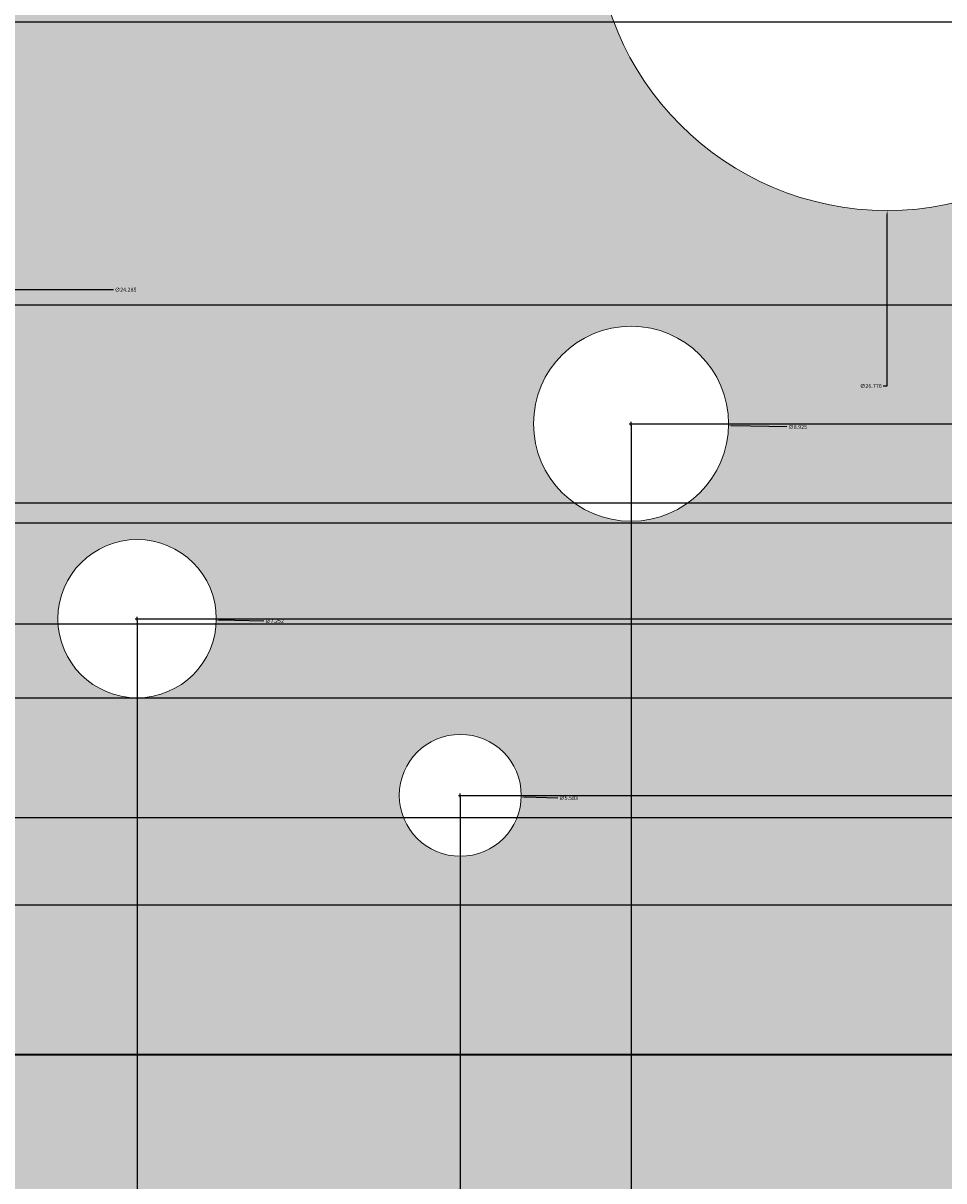
# Model space of a CAD drawing. Units: inches. Extents: x 73 to 607, y 92 to 651.
# Tile 9 of 18: x 504 to 546, y 169 to 222. Entities that reach past the tile are written whole.
import ezdxf

# ---------------------------------------------------------------- set-up
doc = ezdxf.new("R2010")
doc.units = ezdxf.units.IN
doc.header["$MEASUREMENT"] = 0
for name, color, linetype, lineweight in [('A-ANNO-DIMS', 2, 'Continuous', 18), ('A-ELEV', 7, 'Continuous', 35), ('A-ELEV-PANL', 7, 'Continuous', 18), ('A-ELEV-PATT-BKGD', 252, 'Continuous', 13), ('A-ELEV-PATT-SHAD', 8, 'Continuous', 13), ('A-ELEV-PATT-WOOD', 32, 'Continuous', 13)]:
    doc.layers.add(name, color=color, linetype=linetype, lineweight=lineweight)
doc.styles.get("Standard").update_dxf_attribs({"font": 'arial.ttf'})
doc.dimstyles.get("Standard").update_dxf_attribs({"dimtxt": 0.18, "dimasz": 0.18, "dimexe": 0.18, "dimexo": 0.0625, "dimgap": 0.09, "dimtad": 0, "dimtih": 1, "dimtoh": 1, "dimdec": 4, "dimzin": 0, "dimdsep": 46, "dimtxsty": 'Standard', "dimcen": 0.09, "dimadec": 0, "dimazin": 0, "dimtfac": 1, "dimtdec": 4, "dimtofl": 0, "dimtmove": 0, "dimatfit": 3, "dimfxl": 1, "dimtolj": 1, "dimtzin": 0, "dimarcsym": 0})

# ---------------------------------------------------------------- blocks, each defined once
blk = doc.blocks.new('*D15')
at = {"layer": 'A-ANNO-DIMS', "color": 0, "lineweight": -2, "transparency": 16777216}
for p, q in [((454.767, 174.802), (607.278, 174.802)), ((607.098, 174.622), (607.098, 159.185)), ((607.098, 143.384), (607.098, 158.821)), ((580.161, 143.204), (607.278, 143.204))]:
    blk.add_line(p, q, dxfattribs=at)
at = {"layer": 'A-ANNO-DIMS', "color": 0, "transparency": 16777216}
for points in [[(607.068, 174.622), (607.128, 174.622), (607.098, 174.802)], [(607.068, 143.384), (607.128, 143.384), (607.098, 143.204)]]:
    blk.add_solid(points, dxfattribs=at)
at = {"layer": 'Defpoints', "color": 0, "transparency": 16777216}
for p in [(454.705, 174.802), (607.098, 174.802), (580.098, 143.204)]:
    blk.add_point(p, dxfattribs=at)
at = {"layer": 'A-ANNO-DIMS', "color": 0, "transparency": 16777216, "insert": (607.098, 159.003), "char_height": 0.18, "attachment_point": 5}
blk.add_mtext('\\A1;31.6', dxfattribs=at)
blk = doc.blocks.new('*D16')
at = {"layer": 'A-ANNO-DIMS', "color": 0, "lineweight": -2, "transparency": 16777216}
for p, q in [((431.133, 185.662), (607.278, 185.662)), ((607.098, 185.482), (607.098, 180.414)), ((607.098, 174.982), (607.098, 180.05)), ((454.767, 174.802), (607.278, 174.802))]:
    blk.add_line(p, q, dxfattribs=at)
at = {"layer": 'A-ANNO-DIMS', "color": 0, "transparency": 16777216}
for points in [[(607.068, 185.482), (607.128, 185.482), (607.098, 185.662)], [(607.068, 174.982), (607.128, 174.982), (607.098, 174.802)]]:
    blk.add_solid(points, dxfattribs=at)
at = {"layer": 'Defpoints', "color": 0, "transparency": 16777216}
for p in [(431.07, 185.662), (607.098, 185.662), (454.705, 174.802)]:
    blk.add_point(p, dxfattribs=at)
at = {"layer": 'A-ANNO-DIMS', "color": 0, "transparency": 16777216, "insert": (607.098, 180.232), "char_height": 0.18, "attachment_point": 5}
blk.add_mtext('\\A1;10.86', dxfattribs=at)
blk = doc.blocks.new('*D17')
at = {"layer": 'A-ANNO-DIMS', "color": 0, "lineweight": -2, "transparency": 16777216}
for p, q in [((580.161, 262.302), (607.278, 262.302)), ((607.098, 262.122), (607.098, 224.164)), ((607.098, 185.842), (607.098, 223.8)), ((431.133, 185.662), (607.278, 185.662))]:
    blk.add_line(p, q, dxfattribs=at)
at = {"layer": 'A-ANNO-DIMS', "color": 0, "transparency": 16777216}
for points in [[(607.068, 262.122), (607.128, 262.122), (607.098, 262.302)], [(607.068, 185.842), (607.128, 185.842), (607.098, 185.662)]]:
    blk.add_solid(points, dxfattribs=at)
at = {"layer": 'Defpoints', "color": 0, "transparency": 16777216}
for p in [(580.098, 262.302), (607.098, 262.302), (431.07, 185.662)]:
    blk.add_point(p, dxfattribs=at)
at = {"layer": 'A-ANNO-DIMS', "color": 0, "transparency": 16777216, "insert": (607.098, 223.982), "char_height": 0.18, "attachment_point": 5}
blk.add_mtext('\\A1;76.64', dxfattribs=at)
blk = doc.blocks.new('*D62')
at = {"layer": 'A-ANNO-DIMS', "color": 0, "lineweight": -2, "transparency": 16777216}
for p, q in [((488.442, 209.739), (488.442, 209.919)), ((488.352, 209.829), (488.532, 209.829)), ((507.87, 209.829), (500.764, 209.829))]:
    blk.add_line(p, q, dxfattribs=at)
at = {"layer": 'A-ANNO-DIMS', "color": 0, "transparency": 16777216}
blk.add_solid([(500.764, 209.859), (500.764, 209.799), (500.584, 209.829)], dxfattribs=at)
at = {"layer": 'Defpoints', "color": 0, "transparency": 16777216}
for p in [(476.3, 209.828), (500.584, 209.829)]:
    blk.add_point(p, dxfattribs=at)
at = {"layer": 'A-ANNO-DIMS', "color": 0, "transparency": 16777216, "insert": (508.432, 209.829), "char_height": 0.18, "attachment_point": 5}
blk.add_mtext('\\A1;∅24.285', dxfattribs=at)
blk = doc.blocks.new('*D94')
at = {"layer": 'A-ANNO-DIMS', "color": 0, "lineweight": -2, "transparency": 16777216}
for p, q in [((377.023, 209.143), (607.278, 209.143)), ((607.098, 208.963), (607.098, 204.329)), ((607.098, 199.331), (607.098, 203.965)), ((363.319, 199.151), (607.278, 199.151))]:
    blk.add_line(p, q, dxfattribs=at)
at = {"layer": 'A-ANNO-DIMS', "color": 0, "transparency": 16777216}
for points in [[(607.068, 208.963), (607.128, 208.963), (607.098, 209.143)], [(607.068, 199.331), (607.128, 199.331), (607.098, 199.151)]]:
    blk.add_solid(points, dxfattribs=at)
at = {"layer": 'Defpoints', "color": 0, "transparency": 16777216}
for p in [(376.96, 209.143), (363.256, 199.151), (607.098, 199.151)]:
    blk.add_point(p, dxfattribs=at)
at = {"layer": 'A-ANNO-DIMS', "color": 0, "transparency": 16777216, "insert": (607.098, 204.147), "char_height": 0.18, "attachment_point": 5}
blk.add_mtext('\\A1;9.992', dxfattribs=at)
blk = doc.blocks.new('*D95')
at = {"layer": 'A-ANNO-DIMS', "color": 0, "lineweight": -2, "transparency": 16777216}
for p, q in [((363.874, 225.982), (607.278, 225.982)), ((607.098, 225.802), (607.098, 212.749)), ((607.098, 199.331), (607.098, 212.385)), ((363.319, 199.151), (607.278, 199.151))]:
    blk.add_line(p, q, dxfattribs=at)
at = {"layer": 'A-ANNO-DIMS', "color": 0, "transparency": 16777216}
for points in [[(607.068, 225.802), (607.128, 225.802), (607.098, 225.982)], [(607.068, 199.331), (607.128, 199.331), (607.098, 199.151)]]:
    blk.add_solid(points, dxfattribs=at)
at = {"layer": 'Defpoints', "color": 0, "transparency": 16777216}
for p in [(363.812, 225.982), (607.098, 225.982), (363.256, 199.151)]:
    blk.add_point(p, dxfattribs=at)
at = {"layer": 'A-ANNO-DIMS', "color": 0, "transparency": 16777216, "insert": (607.098, 212.567), "char_height": 0.18, "attachment_point": 5}
blk.add_mtext('\\A1;26.83', dxfattribs=at)
blk = doc.blocks.new('*D97')
at = {"layer": 'A-ANNO-DIMS', "color": 0, "lineweight": -2, "transparency": 16777216}
for p, q in [((387.579, 200.076), (607.278, 200.076)), ((607.098, 199.896), (607.098, 197.488)), ((607.098, 194.717), (607.098, 197.125)), ((396.755, 194.537), (607.278, 194.537))]:
    blk.add_line(p, q, dxfattribs=at)
at = {"layer": 'A-ANNO-DIMS', "color": 0, "transparency": 16777216}
for points in [[(607.068, 199.896), (607.128, 199.896), (607.098, 200.076)], [(607.068, 194.717), (607.128, 194.717), (607.098, 194.537)]]:
    blk.add_solid(points, dxfattribs=at)
at = {"layer": 'Defpoints', "color": 0, "transparency": 16777216}
for p in [(387.516, 200.076), (607.098, 200.076), (396.692, 194.537)]:
    blk.add_point(p, dxfattribs=at)
at = {"layer": 'A-ANNO-DIMS', "color": 0, "transparency": 16777216, "insert": (607.098, 197.306), "char_height": 0.18, "attachment_point": 5}
blk.add_mtext('\\A1;5.54', dxfattribs=at)
blk = doc.blocks.new('*D98')
at = {"layer": 'A-ANNO-DIMS', "color": 0, "lineweight": -2, "transparency": 16777216}
for p, q in [((377.023, 209.143), (607.278, 209.143)), ((607.098, 208.963), (607.098, 204.792)), ((607.098, 200.256), (607.098, 204.428)), ((387.579, 200.076), (607.278, 200.076))]:
    blk.add_line(p, q, dxfattribs=at)
at = {"layer": 'A-ANNO-DIMS', "color": 0, "transparency": 16777216}
for points in [[(607.068, 208.963), (607.128, 208.963), (607.098, 209.143)], [(607.068, 200.256), (607.128, 200.256), (607.098, 200.076)]]:
    blk.add_solid(points, dxfattribs=at)
at = {"layer": 'Defpoints', "color": 0, "transparency": 16777216}
for p in [(376.96, 209.143), (607.098, 209.143), (387.516, 200.076)]:
    blk.add_point(p, dxfattribs=at)
at = {"layer": 'A-ANNO-DIMS', "color": 0, "transparency": 16777216, "insert": (607.098, 204.61), "char_height": 0.18, "attachment_point": 5}
blk.add_mtext('\\A1;9.067', dxfattribs=at)
blk = doc.blocks.new('*D99')
at = {"layer": 'A-ANNO-DIMS', "color": 0, "lineweight": -2, "transparency": 16777216}
for p, q in [((373.319, 231.348), (607.278, 231.348)), ((607.098, 231.168), (607.098, 220.428)), ((607.098, 209.323), (607.098, 220.064)), ((377.023, 209.143), (607.278, 209.143))]:
    blk.add_line(p, q, dxfattribs=at)
at = {"layer": 'A-ANNO-DIMS', "color": 0, "transparency": 16777216}
for points in [[(607.068, 231.168), (607.128, 231.168), (607.098, 231.348)], [(607.068, 209.323), (607.128, 209.323), (607.098, 209.143)]]:
    blk.add_solid(points, dxfattribs=at)
at = {"layer": 'Defpoints', "color": 0, "transparency": 16777216}
for p in [(373.257, 231.348), (607.098, 231.348), (376.96, 209.143)]:
    blk.add_point(p, dxfattribs=at)
at = {"layer": 'A-ANNO-DIMS', "color": 0, "transparency": 16777216, "insert": (607.098, 220.246), "char_height": 0.18, "attachment_point": 5}
blk.add_mtext('\\A1;22.205', dxfattribs=at)
blk = doc.blocks.new('*D100')
at = {"layer": 'A-ANNO-DIMS', "color": 0, "lineweight": -2, "transparency": 16777216}
for p, q in [((382.949, 222.096), (607.278, 222.096)), ((607.098, 221.916), (607.098, 211.268)), ((607.098, 200.256), (607.098, 210.904)), ((387.579, 200.076), (607.278, 200.076))]:
    blk.add_line(p, q, dxfattribs=at)
at = {"layer": 'A-ANNO-DIMS', "color": 0, "transparency": 16777216}
for points in [[(607.068, 221.916), (607.128, 221.916), (607.098, 222.096)], [(607.068, 200.256), (607.128, 200.256), (607.098, 200.076)]]:
    blk.add_solid(points, dxfattribs=at)
at = {"layer": 'Defpoints', "color": 0, "transparency": 16777216}
for p in [(382.886, 222.096), (607.098, 222.096), (387.516, 200.076)]:
    blk.add_point(p, dxfattribs=at)
at = {"layer": 'A-ANNO-DIMS', "color": 0, "transparency": 16777216, "insert": (607.098, 211.086), "char_height": 0.18, "attachment_point": 5}
blk.add_mtext('\\A1;22.02', dxfattribs=at)
blk = doc.blocks.new('*D113')
at = {"layer": 'A-ANNO-DIMS', "color": 0, "lineweight": -2, "transparency": 16777216}
for p, q in [((508.958, 194.705), (508.958, 116.024)), ((492.769, 181.596), (492.769, 116.024)), ((492.949, 116.204), (500.478, 116.204)), ((508.778, 116.204), (501.249, 116.204))]:
    blk.add_line(p, q, dxfattribs=at)
at = {"layer": 'A-ANNO-DIMS', "color": 0, "transparency": 16777216}
for points in [[(492.949, 116.234), (492.949, 116.174), (492.769, 116.204)], [(508.778, 116.234), (508.778, 116.174), (508.958, 116.204)]]:
    blk.add_solid(points, dxfattribs=at)
at = {"layer": 'Defpoints', "color": 0, "transparency": 16777216}
for p in [(508.958, 194.767), (492.769, 181.659), (508.958, 116.204)]:
    blk.add_point(p, dxfattribs=at)
at = {"layer": 'A-ANNO-DIMS', "color": 0, "transparency": 16777216, "insert": (500.864, 116.204), "char_height": 0.18, "attachment_point": 5}
blk.add_mtext('\\A1;16.19', dxfattribs=at)
blk = doc.blocks.new('*D114')
at = {"layer": 'A-ANNO-DIMS', "color": 0, "lineweight": -2, "transparency": 16777216}
for p, q in [((508.958, 194.705), (508.958, 116.024)), ((523.753, 186.617), (523.753, 116.024)), ((509.138, 116.204), (515.901, 116.204)), ((523.573, 116.204), (516.81, 116.204))]:
    blk.add_line(p, q, dxfattribs=at)
at = {"layer": 'A-ANNO-DIMS', "color": 0, "transparency": 16777216}
for points in [[(509.138, 116.234), (509.138, 116.174), (508.958, 116.204)], [(523.573, 116.234), (523.573, 116.174), (523.753, 116.204)]]:
    blk.add_solid(points, dxfattribs=at)
at = {"layer": 'Defpoints', "color": 0, "transparency": 16777216}
for p in [(508.958, 194.767), (523.753, 186.679), (523.753, 116.204)]:
    blk.add_point(p, dxfattribs=at)
at = {"layer": 'A-ANNO-DIMS', "color": 0, "transparency": 16777216, "insert": (516.356, 116.204), "char_height": 0.18, "attachment_point": 5}
blk.add_mtext('\\A1;14.794', dxfattribs=at)
blk = doc.blocks.new('*D115')
at = {"layer": 'A-ANNO-DIMS', "color": 0, "lineweight": -2, "transparency": 16777216}
for p, q in [((531.568, 203.63), (531.568, 116.024)), ((523.753, 186.617), (523.753, 116.024)), ((523.933, 116.204), (527.268, 116.204)), ((531.388, 116.204), (528.053, 116.204))]:
    blk.add_line(p, q, dxfattribs=at)
at = {"layer": 'A-ANNO-DIMS', "color": 0, "transparency": 16777216}
for points in [[(523.933, 116.234), (523.933, 116.174), (523.753, 116.204)], [(531.388, 116.234), (531.388, 116.174), (531.568, 116.204)]]:
    blk.add_solid(points, dxfattribs=at)
at = {"layer": 'Defpoints', "color": 0, "transparency": 16777216}
for p in [(531.568, 203.693), (523.753, 186.679), (531.568, 116.204)]:
    blk.add_point(p, dxfattribs=at)
at = {"layer": 'A-ANNO-DIMS', "color": 0, "transparency": 16777216, "insert": (527.661, 116.204), "char_height": 0.18, "attachment_point": 5}
blk.add_mtext('\\A1;7.816', dxfattribs=at)
blk = doc.blocks.new('*D116')
at = {"layer": 'A-ANNO-DIMS', "color": 0, "lineweight": -2, "transparency": 16777216}
for p, q in [((531.568, 203.63), (531.568, 116.024)), ((550.829, 183.548), (550.829, 116.024)), ((531.748, 116.204), (540.814, 116.204)), ((550.649, 116.204), (541.584, 116.204))]:
    blk.add_line(p, q, dxfattribs=at)
at = {"layer": 'A-ANNO-DIMS', "color": 0, "transparency": 16777216}
for points in [[(531.748, 116.234), (531.748, 116.174), (531.568, 116.204)], [(550.649, 116.234), (550.649, 116.174), (550.829, 116.204)]]:
    blk.add_solid(points, dxfattribs=at)
at = {"layer": 'Defpoints', "color": 0, "transparency": 16777216}
for p in [(531.568, 203.693), (550.829, 183.611), (550.829, 116.204)]:
    blk.add_point(p, dxfattribs=at)
at = {"layer": 'A-ANNO-DIMS', "color": 0, "transparency": 16777216, "insert": (541.199, 116.204), "char_height": 0.18, "attachment_point": 5}
blk.add_mtext('\\A1;19.26', dxfattribs=at)
blk = doc.blocks.new('*D120')
at = {"layer": 'A-ANNO-DIMS', "color": 0, "lineweight": -2, "transparency": 16777216}
for p, q in [((468.546, 225.727), (607.278, 225.727)), ((607.098, 225.547), (607.098, 208.616)), ((607.098, 191.322), (607.098, 208.252)), ((469.942, 191.142), (607.278, 191.142))]:
    blk.add_line(p, q, dxfattribs=at)
at = {"layer": 'A-ANNO-DIMS', "color": 0, "transparency": 16777216}
for points in [[(607.068, 225.547), (607.128, 225.547), (607.098, 225.727)], [(607.068, 191.322), (607.128, 191.322), (607.098, 191.142)]]:
    blk.add_solid(points, dxfattribs=at)
at = {"layer": 'Defpoints', "color": 0, "transparency": 16777216}
for p in [(468.484, 225.727), (607.098, 225.727), (469.879, 191.142)]:
    blk.add_point(p, dxfattribs=at)
at = {"layer": 'A-ANNO-DIMS', "color": 0, "transparency": 16777216, "insert": (607.098, 208.434), "char_height": 0.18, "attachment_point": 5}
blk.add_mtext('\\A1;34.585', dxfattribs=at)
blk = doc.blocks.new('*D122')
at = {"layer": 'A-ANNO-DIMS', "color": 0, "lineweight": -2, "transparency": 16777216}
for p, q in [((509.021, 194.767), (607.278, 194.767)), ((607.098, 194.587), (607.098, 188.395)), ((607.098, 181.839), (607.098, 188.031)), ((492.831, 181.659), (607.278, 181.659))]:
    blk.add_line(p, q, dxfattribs=at)
at = {"layer": 'A-ANNO-DIMS', "color": 0, "transparency": 16777216}
for points in [[(607.068, 194.587), (607.128, 194.587), (607.098, 194.767)], [(607.068, 181.839), (607.128, 181.839), (607.098, 181.659)]]:
    blk.add_solid(points, dxfattribs=at)
at = {"layer": 'Defpoints', "color": 0, "transparency": 16777216}
for p in [(508.958, 194.767), (492.769, 181.659), (607.098, 181.659)]:
    blk.add_point(p, dxfattribs=at)
at = {"layer": 'A-ANNO-DIMS', "color": 0, "transparency": 16777216, "insert": (607.098, 188.213), "char_height": 0.18, "attachment_point": 5}
blk.add_mtext('\\A1;13.11', dxfattribs=at)
blk = doc.blocks.new('*D124')
at = {"layer": 'A-ANNO-DIMS', "color": 0, "lineweight": -2, "transparency": 16777216}
for p, q in [((523.815, 186.679), (607.278, 186.679)), ((607.098, 186.499), (607.098, 185.327)), ((607.098, 183.791), (607.098, 184.963)), ((550.891, 183.611), (607.278, 183.611))]:
    blk.add_line(p, q, dxfattribs=at)
at = {"layer": 'A-ANNO-DIMS', "color": 0, "transparency": 16777216}
for points in [[(607.068, 186.499), (607.128, 186.499), (607.098, 186.679)], [(607.068, 183.791), (607.128, 183.791), (607.098, 183.611)]]:
    blk.add_solid(points, dxfattribs=at)
at = {"layer": 'Defpoints', "color": 0, "transparency": 16777216}
for p in [(523.753, 186.679), (607.098, 186.679), (550.829, 183.611)]:
    blk.add_point(p, dxfattribs=at)
at = {"layer": 'A-ANNO-DIMS', "color": 0, "transparency": 16777216, "insert": (607.098, 185.145), "char_height": 0.18, "attachment_point": 5}
blk.add_mtext('\\A1;3.068', dxfattribs=at)
blk = doc.blocks.new('*D125')
at = {"layer": 'A-ANNO-DIMS', "color": 0, "lineweight": -2, "transparency": 16777216}
for p, q in [((509.021, 194.767), (607.278, 194.767)), ((607.098, 194.587), (607.098, 190.905)), ((607.098, 186.859), (607.098, 190.541)), ((523.815, 186.679), (607.278, 186.679))]:
    blk.add_line(p, q, dxfattribs=at)
at = {"layer": 'A-ANNO-DIMS', "color": 0, "transparency": 16777216}
for points in [[(607.068, 194.587), (607.128, 194.587), (607.098, 194.767)], [(607.068, 186.859), (607.128, 186.859), (607.098, 186.679)]]:
    blk.add_solid(points, dxfattribs=at)
at = {"layer": 'Defpoints', "color": 0, "transparency": 16777216}
for p in [(508.958, 194.767), (607.098, 194.767), (523.753, 186.679)]:
    blk.add_point(p, dxfattribs=at)
at = {"layer": 'A-ANNO-DIMS', "color": 0, "transparency": 16777216, "insert": (607.098, 190.723), "char_height": 0.18, "attachment_point": 5}
blk.add_mtext('\\A1;8.088', dxfattribs=at)
blk = doc.blocks.new('*D126')
at = {"layer": 'A-ANNO-DIMS', "color": 0, "lineweight": -2, "transparency": 16777216}
for p, q in [((509.3, 232.7), (607.278, 232.7)), ((607.098, 232.52), (607.098, 213.915)), ((607.098, 194.947), (607.098, 213.552)), ((509.021, 194.767), (607.278, 194.767))]:
    blk.add_line(p, q, dxfattribs=at)
at = {"layer": 'A-ANNO-DIMS', "color": 0, "transparency": 16777216}
for points in [[(607.068, 232.52), (607.128, 232.52), (607.098, 232.7)], [(607.068, 194.947), (607.128, 194.947), (607.098, 194.767)]]:
    blk.add_solid(points, dxfattribs=at)
at = {"layer": 'Defpoints', "color": 0, "transparency": 16777216}
for p in [(509.238, 232.7), (607.098, 232.7), (508.958, 194.767)]:
    blk.add_point(p, dxfattribs=at)
at = {"layer": 'A-ANNO-DIMS', "color": 0, "transparency": 16777216, "insert": (607.098, 213.733), "char_height": 0.18, "attachment_point": 5}
blk.add_mtext('\\A1;37.93', dxfattribs=at)
blk = doc.blocks.new('*D127')
at = {"layer": 'A-ANNO-DIMS', "color": 0, "lineweight": -2, "transparency": 16777216}
for p, q in [((524.094, 250.271), (607.278, 250.271)), ((607.098, 250.091), (607.098, 218.657)), ((607.098, 186.859), (607.098, 218.293)), ((523.815, 186.679), (607.278, 186.679))]:
    blk.add_line(p, q, dxfattribs=at)
at = {"layer": 'A-ANNO-DIMS', "color": 0, "transparency": 16777216}
for points in [[(607.068, 250.091), (607.128, 250.091), (607.098, 250.271)], [(607.068, 186.859), (607.128, 186.859), (607.098, 186.679)]]:
    blk.add_solid(points, dxfattribs=at)
at = {"layer": 'Defpoints', "color": 0, "transparency": 16777216}
for p in [(524.032, 250.271), (607.098, 250.271), (523.753, 186.679)]:
    blk.add_point(p, dxfattribs=at)
at = {"layer": 'A-ANNO-DIMS', "color": 0, "transparency": 16777216, "insert": (607.098, 218.475), "char_height": 0.18, "attachment_point": 5}
blk.add_mtext('\\A1;63.59', dxfattribs=at)
blk = doc.blocks.new('*D128')
at = {"layer": 'A-ANNO-DIMS', "color": 0, "lineweight": -2, "transparency": 16777216}
for p, q in [((531.631, 203.693), (607.278, 203.693)), ((607.098, 203.513), (607.098, 195.368)), ((607.098, 186.859), (607.098, 195.004)), ((523.815, 186.679), (607.278, 186.679))]:
    blk.add_line(p, q, dxfattribs=at)
at = {"layer": 'A-ANNO-DIMS', "color": 0, "transparency": 16777216}
for points in [[(607.068, 203.513), (607.128, 203.513), (607.098, 203.693)], [(607.068, 186.859), (607.128, 186.859), (607.098, 186.679)]]:
    blk.add_solid(points, dxfattribs=at)
at = {"layer": 'Defpoints', "color": 0, "transparency": 16777216}
for p in [(531.568, 203.693), (607.098, 203.693), (523.753, 186.679)]:
    blk.add_point(p, dxfattribs=at)
at = {"layer": 'A-ANNO-DIMS', "color": 0, "transparency": 16777216, "insert": (607.098, 195.186), "char_height": 0.18, "attachment_point": 5}
blk.add_mtext('\\A1;17.014', dxfattribs=at)
blk = doc.blocks.new('*D159')
at = {"layer": 'A-ANNO-DIMS', "color": 0, "lineweight": -2, "transparency": 16777216}
for p, q in [((543.292, 226.752), (543.292, 226.932)), ((543.202, 226.842), (543.382, 226.842)), ((543.289, 205.422), (543.29, 213.275)), ((543.109, 205.422), (543.289, 205.422))]:
    blk.add_line(p, q, dxfattribs=at)
at = {"layer": 'A-ANNO-DIMS', "color": 0, "transparency": 16777216}
blk.add_solid([(543.26, 213.275), (543.32, 213.275), (543.29, 213.455)], dxfattribs=at)
at = {"layer": 'Defpoints', "color": 0, "transparency": 16777216}
for p in [(543.294, 240.23), (543.29, 213.455)]:
    blk.add_point(p, dxfattribs=at)
at = {"layer": 'A-ANNO-DIMS', "color": 0, "transparency": 16777216, "insert": (542.547, 205.422), "char_height": 0.18, "attachment_point": 5}
blk.add_mtext('\\A1;∅26.776', dxfattribs=at)
blk = doc.blocks.new('*D162')
at = {"layer": 'A-ANNO-DIMS', "color": 0, "lineweight": -2, "transparency": 16777216}
for p, q in [((531.478, 203.693), (531.658, 203.693)), ((531.568, 203.603), (531.568, 203.783)), ((538.707, 203.545), (536.21, 203.597))]:
    blk.add_line(p, q, dxfattribs=at)
at = {"layer": 'A-ANNO-DIMS', "color": 0, "transparency": 16777216}
blk.add_solid([(536.211, 203.627), (536.209, 203.567), (536.03, 203.6)], dxfattribs=at)
at = {"layer": 'Defpoints', "color": 0, "transparency": 16777216}
for p in [(527.107, 203.785), (536.03, 203.6)]:
    blk.add_point(p, dxfattribs=at)
at = {"layer": 'A-ANNO-DIMS', "color": 0, "transparency": 16777216, "insert": (539.199, 203.545), "char_height": 0.18, "attachment_point": 5}
blk.add_mtext('\\A1;∅8.925', dxfattribs=at)
blk = doc.blocks.new('*D164')
at = {"layer": 'A-ANNO-DIMS', "color": 0, "lineweight": -2, "transparency": 16777216}
for p, q in [((508.868, 194.767), (509.048, 194.767)), ((508.958, 194.677), (508.958, 194.857)), ((514.759, 194.661), (512.764, 194.698))]:
    blk.add_line(p, q, dxfattribs=at)
at = {"layer": 'A-ANNO-DIMS', "color": 0, "transparency": 16777216}
blk.add_solid([(512.764, 194.728), (512.763, 194.668), (512.584, 194.701)], dxfattribs=at)
at = {"layer": 'Defpoints', "color": 0, "transparency": 16777216}
for p in [(505.333, 194.834), (512.584, 194.701)]:
    blk.add_point(p, dxfattribs=at)
at = {"layer": 'A-ANNO-DIMS', "color": 0, "transparency": 16777216, "insert": (515.25, 194.661), "char_height": 0.18, "attachment_point": 5}
blk.add_mtext('\\A1;∅7.252', dxfattribs=at)
blk = doc.blocks.new('*D167')
at = {"layer": 'A-ANNO-DIMS', "color": 0, "lineweight": -2, "transparency": 16777216}
for p, q in [((523.663, 186.679), (523.843, 186.679)), ((523.753, 186.589), (523.753, 186.769)), ((528.217, 186.556), (526.723, 186.597))]:
    blk.add_line(p, q, dxfattribs=at)
at = {"layer": 'A-ANNO-DIMS', "color": 0, "transparency": 16777216}
blk.add_solid([(526.724, 186.627), (526.722, 186.567), (526.543, 186.602)], dxfattribs=at)
at = {"layer": 'Defpoints', "color": 0, "transparency": 16777216}
for p in [(520.962, 186.756), (526.543, 186.602)]:
    blk.add_point(p, dxfattribs=at)
at = {"layer": 'A-ANNO-DIMS', "color": 0, "transparency": 16777216, "insert": (528.709, 186.556), "char_height": 0.18, "attachment_point": 5}
blk.add_mtext('\\A1;∅5.583', dxfattribs=at)

msp = doc.modelspace()

# ---------------------------------------------------------------- hatches: boundary and pattern name
at = {"layer": 'A-ELEV-PATT-BKGD'}
h = msp.add_hatch(color=256, dxfattribs=at)
h.dxf.hatch_style = 1
h.paths.add_polyline_path([(321.3008, 479.2042), (312.3008, 479.2042), (312.3008, 478.7576), (312.3008, 412.636), (321.3008, 412.636)])
h.paths.add_polyline_path([(312.3008, 504.7576), (256.4726, 504.7576), (256.4726, 503.4576), (312.3008, 503.4576)], flags=17)
h.paths.add_polyline_path([(321.3008, 543.1576), (321.3008, 552.1576), (320.3257, 552.1576), (312.3008, 552.1576), (256.4726, 552.1576), (256.4726, 543.1576), (312.3008, 543.1576), (312.3008, 479.2042), (321.3008, 479.2042)])
h.paths.add_polyline_path([(451.5214, 412.636), (256.4726, 412.636), (256.4726, 403.636), (442.5214, 403.636), (442.5214, 320.2042), (206.1343, 320.2042), (206.1343, 320.9135), (206.1343, 403.636), (256.4726, 403.636), (256.4726, 412.636), (201.6343, 412.636), (201.6343, 320.9135), (201.6343, 320.2042), (201.6343, 311.2042), (256.4726, 311.2042), (451.5214, 311.2042)])
h.paths.add_polyline_path([(431.07, 258.6914), (369.5339, 258.6914), (369.5339, 247.4054), (396.692, 247.4054), (425.07, 247.4054), (425.07, 194.7312), (396.692, 194.6197), (396.692, 194.5366), (369.5339, 194.5366), (369.5339, 185.6619), (431.07, 185.6619)])
h.paths.add_polyline_path([(580.0983, 262.3024), (451.5214, 262.3024), (451.5214, 143.2042), (580.0983, 143.2042)])
h.paths.add_polyline_path([(454.7049, 174.802), (454.7049, 256.6321), (577.9249, 256.6321), (577.9249, 174.802)], flags=16)
h.paths.add_polyline_path([(465.9716, 191.1416, -1), (473.7874, 191.1416, -1)], flags=0)
h.paths.add_polyline_path([(490.5373, 181.6586, -1), (494.9999, 181.6586, -1)], flags=0)
h.paths.add_polyline_path([(476.2996, 209.8287, -1), (500.5844, 209.8287, -1)], flags=0)
h.paths.add_polyline_path([(505.3326, 194.7675, -1), (512.5843, 194.7675, -1)], flags=0)
h.paths.add_polyline_path([(520.9613, 186.679, -1), (526.544, 186.679, -1)], flags=0)
h.paths.add_polyline_path([(466.8103, 225.7267, -1), (470.1573, 225.7267, -1)], flags=0)
h.paths.add_polyline_path([(527.1059, 203.6926, -1), (536.0311, 203.6926, -1)], flags=0)
h.paths.add_polyline_path([(504.775, 232.6995, -1), (513.7002, 232.6995, -1)], flags=0)
h.paths.add_polyline_path([(546.9241, 183.611, -1), (554.7336, 183.611, -1)], flags=0)
h.paths.add_polyline_path([(459.5544, 243.856, -1), (466.8061, 243.856, -1)], flags=0)
h.paths.add_polyline_path([(476.3045, 246.924, -1), (488.5767, 246.924, -1)], flags=0)
h.paths.add_polyline_path([(529.9044, 226.8424, -1), (556.68, 226.8424, -1)], flags=0)
h.paths.add_polyline_path([(554.1814, 203.9716, -1), (561.4331, 203.9716, -1)], flags=0)
h.paths.add_polyline_path([(567.8561, 193.3729, -1), (570.6475, 193.3729, -1)], flags=0)
h.paths.add_polyline_path([(522.3584, 250.271, -1), (525.7053, 250.271, -1)], flags=0)
h.paths.add_polyline_path([(561.9965, 245.2506, -1), (567.5748, 245.2506, -1)], flags=0)
h.paths.add_polyline_path([(347.8686, 194.5366), (341.8686, 194.5366), (341.8686, 194.5452), (314.0144, 194.5452), (314.0144, 188.5452), (347.8686, 188.5452)])
h.paths.add_polyline_path([(347.8686, 253.4054), (314.0144, 253.4054), (314.0144, 247.4054), (341.8686, 247.4054), (347.8686, 247.4054)])
h.paths.add_polyline_path([(304.3559, 253.4054), (298.3559, 253.4054), (298.3559, 188.5452), (304.3559, 188.5452)])
h.paths.add_polyline_path([(450.6603, 552.1576), (369.9727, 552.1576), (369.9727, 479.2042), (374.4727, 479.2042), (374.4727, 547.6576), (446.1603, 547.6576), (446.1603, 479.2042), (450.6603, 479.2042)])
h.paths.add_polyline_path([(374.4727, 479.2042), (369.9727, 479.2042), (369.9727, 465.0632), (374.4727, 465.0632)])
h.paths.add_polyline_path([(450.6603, 479.2042), (446.1603, 479.2042), (446.1603, 465.0632), (450.6603, 465.0632)])
h.paths.add_polyline_path([(256.4726, 281.6039), (109.0983, 281.6039), (100.0983, 281.6039), (100.0983, 167.2042), (100.0983, 143.2042), (109.0983, 143.2042), (109.0983, 167.2042), (109.0983, 272.6039), (256.4726, 272.6039)])
at = {"layer": 'A-ELEV-PATT-SHAD'}
h = msp.add_hatch(color=256, dxfattribs=at)
h.dxf.hatch_style = 1
h.paths.add_polyline_path([(451.5214, 412.636), (256.4726, 412.636), (256.4726, 403.636), (442.5214, 403.636), (442.5214, 320.2042), (206.1343, 320.2042), (206.1343, 320.9135), (206.1343, 403.636), (256.4726, 403.636), (256.4726, 412.636), (201.6343, 412.636), (201.6343, 320.9135), (201.6343, 320.2042), (201.6343, 311.2042), (256.4726, 311.2042), (451.5214, 311.2042)])
h.paths.add_polyline_path([(580.0983, 262.3024), (451.5214, 262.3024), (451.5214, 143.2042), (580.0983, 143.2042)])
h.paths.add_polyline_path([(454.7049, 174.802), (454.7049, 256.6321), (577.9249, 256.6321), (577.9249, 174.802)], flags=16)
h.paths.add_polyline_path([(465.9716, 191.1416, -1), (473.7874, 191.1416, -1)], flags=0)
h.paths.add_polyline_path([(490.5373, 181.6586, -1), (494.9999, 181.6586, -1)], flags=0)
h.paths.add_polyline_path([(476.2996, 209.8287, -1), (500.5844, 209.8287, -1)], flags=0)
h.paths.add_polyline_path([(505.3326, 194.7675, -1), (512.5843, 194.7675, -1)], flags=0)
h.paths.add_polyline_path([(520.9613, 186.679, -1), (526.544, 186.679, -1)], flags=0)
h.paths.add_polyline_path([(466.8103, 225.7267, -1), (470.1573, 225.7267, -1)], flags=0)
h.paths.add_polyline_path([(527.1059, 203.6926, -1), (536.0311, 203.6926, -1)], flags=0)
h.paths.add_polyline_path([(459.5544, 243.856, -1), (466.8061, 243.856, -1)], flags=0)
h.paths.add_polyline_path([(504.775, 232.6995, -1), (513.7002, 232.6995, -1)], flags=0)
h.paths.add_polyline_path([(476.3045, 246.924, -1), (488.5767, 246.924, -1)], flags=0)
h.paths.add_polyline_path([(546.9241, 183.611, -1), (554.7336, 183.611, -1)], flags=0)
h.paths.add_polyline_path([(529.9044, 226.8424, -1), (556.68, 226.8424, -1)], flags=0)
h.paths.add_polyline_path([(554.1814, 203.9716, -1), (561.4331, 203.9716, -1)], flags=0)
h.paths.add_polyline_path([(522.3584, 250.271, -1), (525.7053, 250.271, -1)], flags=0)
h.paths.add_polyline_path([(567.8561, 193.3729, -1), (570.6475, 193.3729, -1)], flags=0)
h.paths.add_polyline_path([(561.9965, 245.2506, -1), (567.5748, 245.2506, -1)], flags=0)
h.paths.add_polyline_path([(431.07, 258.6914), (369.5339, 258.6914), (369.5339, 247.4054), (396.692, 247.4054), (425.07, 247.4054), (425.07, 194.7312), (396.692, 194.6197), (396.692, 194.5366), (369.5339, 194.5366), (369.5339, 185.6619), (431.07, 185.6619)])
h.paths.add_polyline_path([(347.8686, 253.4054), (314.0144, 253.4054), (314.0144, 247.4054), (341.8686, 247.4054), (347.8686, 247.4054)])
h.paths.add_polyline_path([(304.3559, 253.4054), (298.3559, 253.4054), (298.3559, 188.5452), (304.3559, 188.5452)])
h.paths.add_polyline_path([(347.8686, 194.5366), (341.8686, 194.5366), (341.8686, 194.5452), (314.0144, 194.5452), (314.0144, 188.5452), (347.8686, 188.5452)])
at = {"layer": 'A-ELEV-PATT-WOOD'}
h = msp.add_hatch(color=256, dxfattribs=at)
h.dxf.hatch_style = 1
h.paths.add_polyline_path([(577.9249, 256.6321), (454.7049, 256.6321), (454.7049, 174.802), (577.9249, 174.802)])
h.paths.add_polyline_path([(476.2996, 209.8287, -1), (500.5844, 209.8287, -1)], flags=16)
h.paths.add_polyline_path([(473.7874, 191.1416, -1), (465.9716, 191.1416, -1)], flags=16)
h.paths.add_polyline_path([(466.8103, 225.7267, -1), (470.1573, 225.7267, -1)], flags=16)
h.paths.add_polyline_path([(459.5544, 243.856, -1), (466.8061, 243.856, -1)], flags=16)
h.paths.add_polyline_path([(494.9999, 181.6586, -1), (490.5373, 181.6586, -1)], flags=16)
h.paths.add_polyline_path([(476.3045, 246.924, -1), (488.5767, 246.924, -1)], flags=16)
h.paths.add_polyline_path([(512.5843, 194.7675, -1), (505.3326, 194.7675, -1)], flags=16)
h.paths.add_polyline_path([(504.775, 232.6995, -1), (513.7002, 232.6995, -1)], flags=16)
h.paths.add_polyline_path([(526.544, 186.679, -1), (520.9613, 186.679, -1)], flags=16)
h.paths.add_polyline_path([(536.0311, 203.6926, -1), (527.1059, 203.6926, -1)], flags=16)
h.paths.add_polyline_path([(529.9044, 226.8424, -1), (556.68, 226.8424, -1)], flags=16)
h.paths.add_polyline_path([(522.3584, 250.271, -1), (525.7053, 250.271, -1)], flags=16)
h.paths.add_polyline_path([(554.7336, 183.611, -1), (546.9241, 183.611, -1)], flags=16)
h.paths.add_polyline_path([(561.4331, 203.9716, -1), (554.1814, 203.9716, -1)], flags=16)
h.paths.add_polyline_path([(561.9965, 245.2506, -1), (567.5748, 245.2506, -1)], flags=16)
h.paths.add_polyline_path([(570.6475, 193.3729, -1), (567.8561, 193.3729, -1)], flags=16)

# ---------------------------------------------------------------- linework, layer by layer
at = {"layer": 'A-ELEV'}
msp.add_lwpolyline([(454.7049, 256.6321), (577.9249, 256.6321), (577.9249, 174.802), (454.7049, 174.802)], close=True, dxfattribs=at)
at = {"layer": 'A-ELEV-PANL'}
for centre, radius in [((543.2922, 226.8424), 13.3878), ((531.5685, 203.6926), 4.4626), ((508.9585, 194.7675), 3.6259), ((523.7527, 186.679), 2.7914)]:
    msp.add_circle(centre, radius, dxfattribs=at)

# ---------------------------------------------------------------- dimensions: what is measured, and where the dimension line sits
at = {"layer": 'A-ANNO-DIMS'}
for base, p1, p2, override, picture, middle in [((607.0983, 262.3024), (431.07, 185.6619), (580.0983, 262.3024), {"dimdec": 2, "dimlfac": 1, "dimrnd": 0, "dimzin": 0, "dimdsep": 46, "dimlunit": 2}, '*D17', (607.0983, 223.9821)), ((607.0983, 250.271), (523.7527, 186.679), (524.0318, 250.271), {"dimdec": 2, "dimlfac": 1, "dimrnd": 0, "dimzin": 0, "dimdsep": 46, "dimlunit": 2}, '*D127', (607.0983, 218.475)), ((607.0983, 232.6995), (508.9585, 194.7675), (509.2376, 232.6995), {"dimdec": 2, "dimlfac": 1, "dimrnd": 0, "dimzin": 0, "dimdsep": 46, "dimlunit": 2}, '*D126', (607.0983, 213.7335)), ((607.0983, 231.3482), (376.9603, 209.1433), (373.2566, 231.3482), {"dimdec": 3, "dimlfac": 1, "dimrnd": 0, "dimzin": 0, "dimdsep": 46, "dimlunit": 2}, '*D99', (607.0983, 220.2458)), ((607.0983, 225.982), (363.2564, 199.1512), (363.8119, 225.982), {"dimdec": 2, "dimlfac": 1, "dimrnd": 0, "dimzin": 0, "dimdsep": 46, "dimlunit": 2}, '*D95', (607.0983, 212.5666)), ((607.0983, 225.7267), (469.8795, 191.1416), (468.4838, 225.7267), {"dimdec": 3, "dimlfac": 1, "dimrnd": 0, "dimzin": 0, "dimdsep": 46, "dimlunit": 2}, '*D120', (607.0983, 208.4342)), ((607.0983, 222.0962), (387.5161, 200.0764), (382.8864, 222.0962), {"dimdec": 2, "dimlfac": 1, "dimrnd": 0, "dimzin": 0, "dimdsep": 46, "dimlunit": 2}, '*D100', (607.0983, 211.0863)), ((607.0983, 199.1512), (376.9603, 209.1433), (363.2564, 199.1512), {"dimdec": 3, "dimlfac": 1, "dimrnd": 0, "dimzin": 0, "dimdsep": 46, "dimlunit": 2}, '*D94', (607.0983, 204.1472)), ((607.0983, 209.1433), (387.5161, 200.0764), (376.9603, 209.1433), {"dimdec": 3, "dimlfac": 1, "dimrnd": 0, "dimzin": 0, "dimdsep": 46, "dimlunit": 2}, '*D98', (607.0983, 204.6098)), ((607.0983, 203.6926), (523.7527, 186.679), (531.5685, 203.6926), {"dimdec": 3, "dimlfac": 1, "dimrnd": 0, "dimzin": 0, "dimdsep": 46, "dimlunit": 2}, '*D128', (607.0983, 195.1858)), ((607.0983, 200.0764), (396.692, 194.5366), (387.5161, 200.0764), {"dimdec": 2, "dimlfac": 1, "dimrnd": 0, "dimzin": 0, "dimdsep": 46, "dimlunit": 2}, '*D97', (607.0983, 197.3065)), ((607.0983, 181.6586), (508.9585, 194.7675), (492.7686, 181.6586), {"dimdec": 2, "dimlfac": 1, "dimrnd": 0, "dimzin": 0, "dimdsep": 46, "dimlunit": 2}, '*D122', (607.0983, 188.213)), ((607.0983, 194.76746), (523.75269, 186.679), (508.95849, 194.76746), {"dimdec": 3, "dimlfac": 1, "dimrnd": 0, "dimzin": 0, "dimdsep": 46, "dimlunit": 2}, '*D125', (607.0983, 190.72323)), ((607.0983, 186.679), (550.8289, 183.611), (523.7527, 186.679), {"dimdec": 3, "dimlfac": 1, "dimrnd": 0, "dimzin": 0, "dimdsep": 46, "dimlunit": 2}, '*D124', (607.0983, 185.145)), ((607.0983, 185.6619), (454.7049, 174.802), (431.07, 185.6619), {"dimdec": 2, "dimlfac": 1, "dimrnd": 0, "dimzin": 0, "dimdsep": 46, "dimlunit": 2}, '*D16', (607.0983, 180.232)), ((607.0983, 174.802), (580.0983, 143.2042), (454.7049, 174.802), {"dimdec": 1, "dimlfac": 1, "dimrnd": 0, "dimzin": 0, "dimdsep": 46, "dimlunit": 2}, '*D15', (607.0983, 159.0031))]:
    dim = msp.add_linear_dim(base=base, p1=p1, p2=p2, angle=90, dimstyle='Standard', override=override, dxfattribs=at)
    dim.commit()
    dim.dimension.update_dxf_attribs({"geometry": picture, "text_midpoint": middle})
for p1, p2, picture, middle in [((543.2944, 240.2301), (543.29, 213.4546), '*D159', (542.5472, 205.4219)), ((476.2996, 209.8284), (500.5844, 209.829), '*D62', (507.8699, 209.8292)), ((527.1068, 203.7849), (536.0301, 203.6004), '*D162', (538.7071, 203.5451)), ((505.3332, 194.8341), (512.5837, 194.7009), '*D164', (514.7589, 194.6609)), ((520.9624, 186.7562), (526.543, 186.6019), '*D167', (528.2172, 186.5556))]:
    dim = msp.add_diameter_dim_2p(p1=p1, p2=p2, dimstyle='Standard', override={"dimdec": 3, "dimlfac": 1, "dimrnd": 0, "dimzin": 0, "dimdsep": 46, "dimlunit": 2}, dxfattribs=at)
    dim.commit()
    dim.dimension.update_dxf_attribs({"geometry": picture, "text_midpoint": middle, "dimtype": 163})
for base, p1, p2, override, picture, middle in [((531.5685, 116.2042), (523.7527, 186.679), (531.5685, 203.6926), {"dimdec": 3, "dimlfac": 1, "dimrnd": 0, "dimzin": 0, "dimdsep": 46, "dimlunit": 2}, '*D115', (527.6606, 116.2042)), ((550.8289, 116.2042), (531.5685, 203.6926), (550.8289, 183.611), {"dimdec": 2, "dimlfac": 1, "dimrnd": 0, "dimzin": 0, "dimdsep": 46, "dimlunit": 2}, '*D116', (541.1987, 116.2042)), ((508.9585, 116.2042), (492.7686, 181.6586), (508.9585, 194.7675), {"dimdec": 2, "dimlfac": 1, "dimrnd": 0, "dimzin": 0, "dimdsep": 46, "dimlunit": 2}, '*D113', (500.8636, 116.2042)), ((523.7527, 116.2042), (508.9585, 194.7675), (523.7527, 186.679), {"dimdec": 3, "dimlfac": 1, "dimrnd": 0, "dimzin": 0, "dimdsep": 46, "dimlunit": 2}, '*D114', (516.3556, 116.2042))]:
    dim = msp.add_linear_dim(base=base, p1=p1, p2=p2, dimstyle='Standard', override=override, dxfattribs=at)
    dim.commit()
    dim.dimension.update_dxf_attribs({"geometry": picture, "text_midpoint": middle})

doc.saveas('drawing.dxf')
